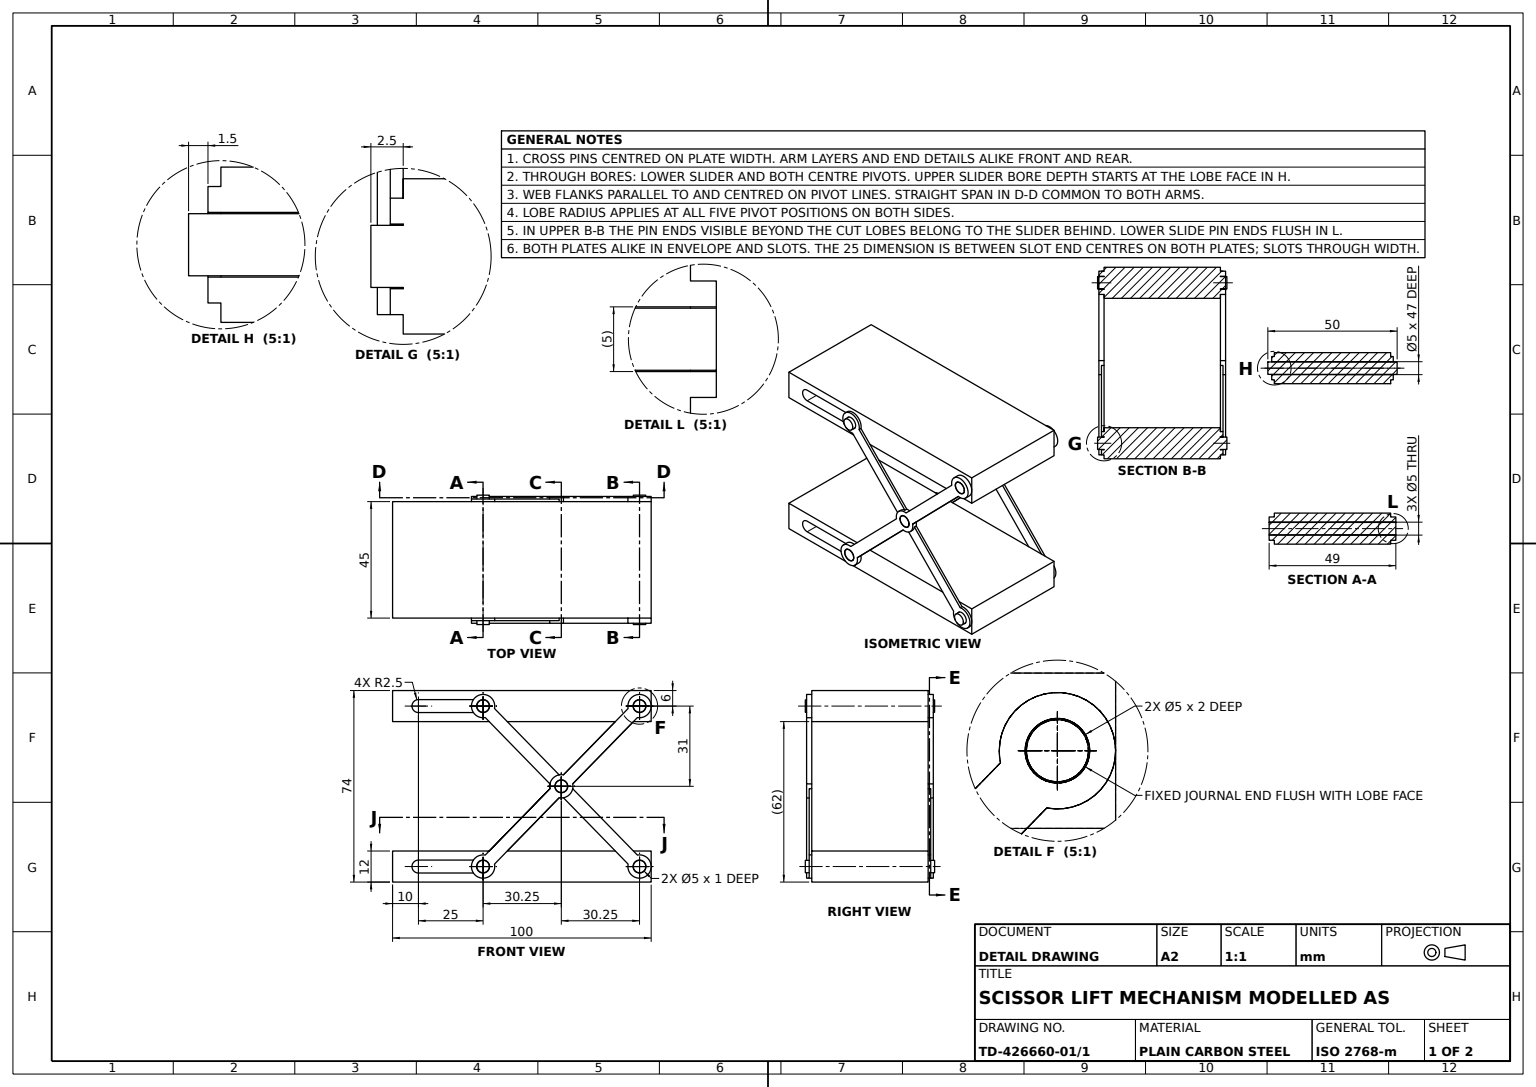
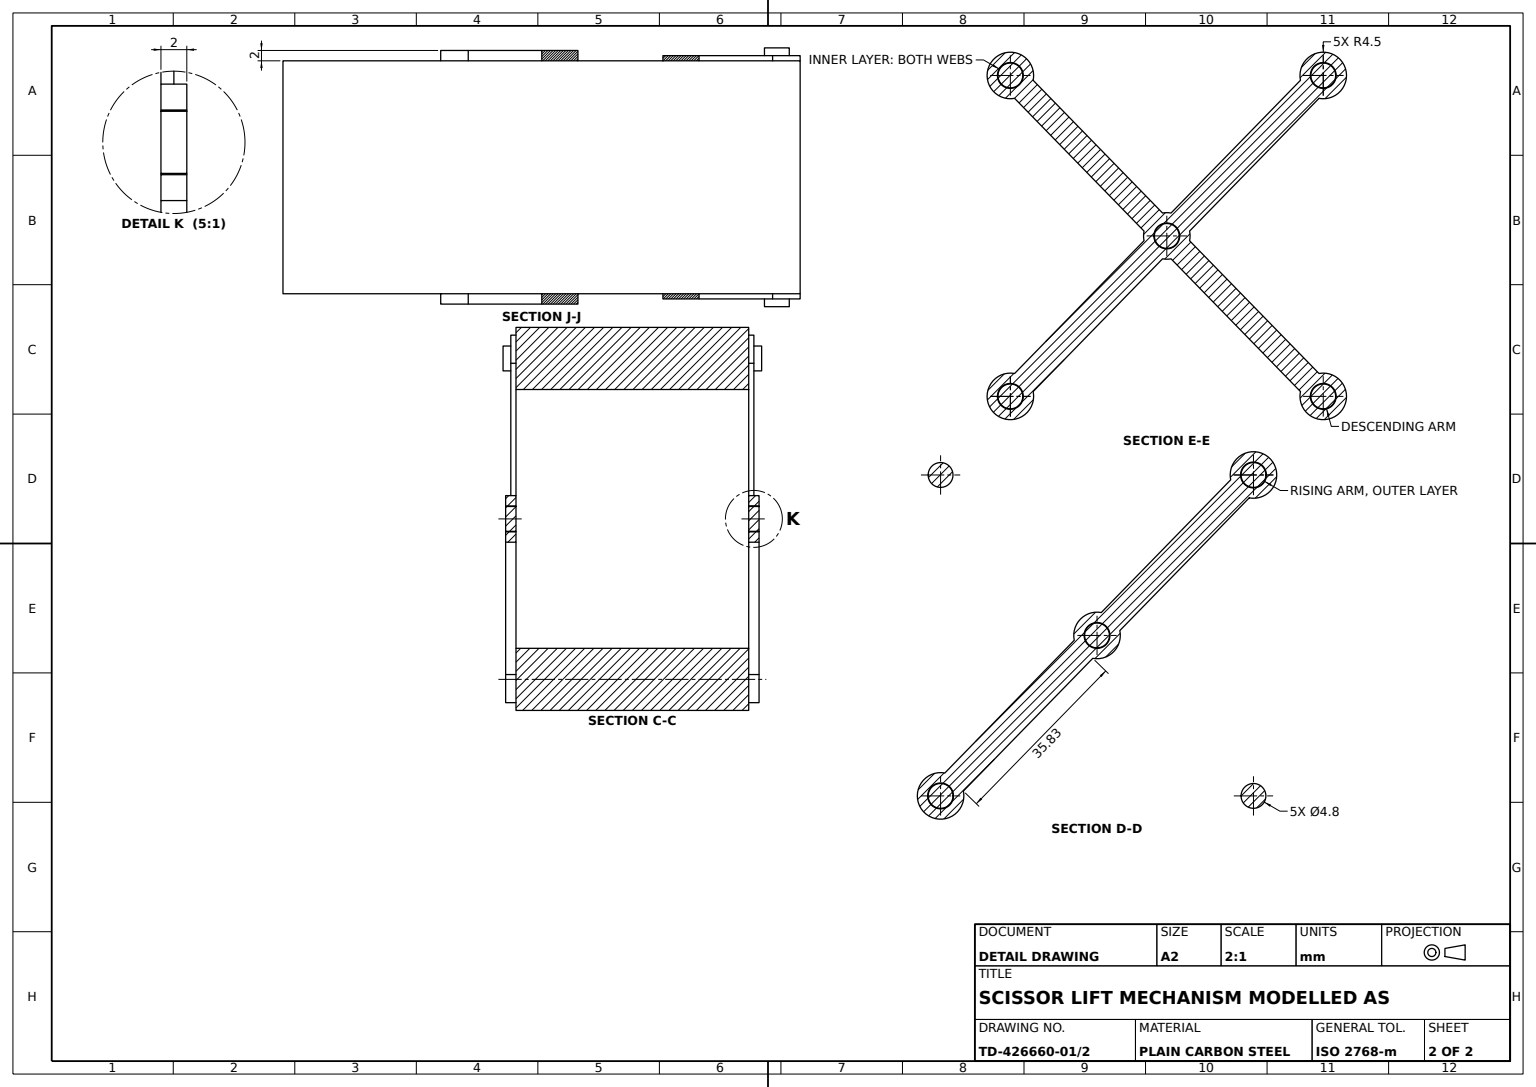
from build123d import *
from build123d.topology import SkipClean

# Parameters (mm, degrees)
BASE_PLATE_SKETCH_W              = 100
BASE_PLATE_SKETCH_H              = 45
BASE_PLATE_DEPTH                 = 12
BASE_PLATE_GUIDE_SLOT_DEPTH      = 200
TOP_PLATE_SKETCH_W               = 100
TOP_PLATE_SKETCH_H               = 45
TOP_PLATE_DEPTH                  = 12
TOP_PLATE_GUIDE_SLOT_DEPTH       = 50
FRONT_SCISSOR_ARM_A_SKETCH_R     = 2.5
FRONT_SCISSOR_ARM_A_DEPTH        = 1
FRONT_SCISSOR_ARM_B_SKETCH_R     = 2.5
FRONT_SCISSOR_ARM_B_DEPTH        = 2
FRONT_START                      = -2
FRONT_ARM_LINK_PIN_SKETCH_R      = 4.5
FRONT_ARM_LINK_PIN_SKETCH_R_2    = 2.5
FRONT_ARM_LINK_PIN_DEPTH         = 2
CENTER_PIVOT_PIN_FRONT_SKETCH_R  = 2.4
CENTER_PIVOT_PIN_FRONT_4_8_DEPTH = 2
LOWER_CROSS_PIN_SKETCH_R         = 2.4
LOWER_CROSS_PIN_4_8X49_DEPTH     = 49
UPPER_CROSS_PIN_HEAD_SKETCH_R    = 2.4
UPPER_CROSS_PIN_HEAD_DEPTH       = 1.5
UPPER_CROSS_PIN_SKETCH_R         = 2.4
UPPER_CROSS_PIN_4_8X47_5_DEPTH   = 47.5
FRONT_ARM_PIN_SKETCH_R           = 2.4
FRONT_ARM_PIN_4_8_DEPTH          = 2
LOWER_ROLLER_PIN_SKETCH_R        = 2.4
LOWER_ROLLER_PIN_4_8_DEPTH       = 2.5
REAR_START                       = 1
REAR_SCISSOR_ARM_A_SKETCH_R      = 2.5
REAR_SCISSOR_ARM_A_DEPTH         = 1
UPPER_START                      = 2.5
UPPER_CROSS_PIN_END_SKETCH_R     = 2.4
UPPER_CROSS_PIN_END_4_8_DEPTH    = 2.5
REAR_START_2                     = 2
REAR_SCISSOR_ARM_B_SKETCH_R      = 2.5
REAR_SCISSOR_ARM_B_DEPTH         = 2
CENTER_PIVOT_PIN_REAR_SKETCH_R   = 2.4
CENTER_PIVOT_PIN_REAR_4_8_DEPTH  = 2
REAR_ARM_PIN_SKETCH_R            = 2.4
REAR_ARM_PIN_4_8_DEPTH           = 2


with BuildPart() as part:
    # Base Plate Sketch → Base Plate (new body)
    with BuildSketch(Plane(origin=(0, 0, 0), x_dir=(1, 0, 0), z_dir=(0, 1, 0))):
        Rectangle(BASE_PLATE_SKETCH_W, BASE_PLATE_SKETCH_H)
    extrude(amount=BASE_PLATE_DEPTH)

    # Base Plate Guide Slot Sketch → Base Plate Guide Slot (cut)
    with BuildSketch(Plane.XY.offset(22.5)):
        with BuildLine():
            Line((-15, 3.5), (-40, 3.5))
            ThreePointArc((-40, 3.5), (-42.5, 6), (-40, 8.5))
            Line((-40, 8.5), (-15, 8.5))
            ThreePointArc((-15, 8.5), (-12.5, 6), (-15, 3.5))
        make_face()
    extrude(amount=-BASE_PLATE_GUIDE_SLOT_DEPTH, mode=Mode.SUBTRACT)



with BuildPart() as body_2:
    # Top Plate Sketch → Top Plate (new body)
    with BuildSketch(Plane(origin=(0, 62, 0), x_dir=(1, 0, 0), z_dir=(0, 1, 0))):
        Rectangle(TOP_PLATE_SKETCH_W, TOP_PLATE_SKETCH_H)
    extrude(amount=TOP_PLATE_DEPTH)

    # Top Plate Guide Slot Sketch → Top Plate Guide Slot (cut)
    with BuildSketch(Plane.XY.offset(22.5)):
        with BuildLine():
            Line((-15, 65.5), (-40, 65.5))
            ThreePointArc((-40, 65.5), (-42.5, 68), (-40, 70.5))
            Line((-40, 70.5), (-15, 70.5))
            ThreePointArc((-15, 70.5), (-12.5, 68), (-15, 65.5))
        make_face()
    extrude(amount=-TOP_PLATE_GUIDE_SLOT_DEPTH, mode=Mode.SUBTRACT)


with BuildPart() as part_1:
    with SkipClean():  # the faces are left unmerged after this step: merging them gives an invalid solid
        add(part.part)

        add(body_2.part)  # Front Scissor Arm A merges body 2
        # Front Scissor Arm A Sketch → Front Scissor Arm A (add)
        with BuildSketch(Plane.XY.offset(22.5)):
            with BuildLine():
                Line((-14.176120486, 63.576062552), (10.847562598, 37.931957574))
                ThreePointArc((10.847562598, 37.931957574), (12.029297901, 33.857218113), (16.073879514, 32.576062552))
                Line((16.073879514, 32.576062552), (41.097562598, 6.931957574))
                ThreePointArc((41.097562598, 6.931957574), (48.642781887, 2.779297901), (44.676120486, 10.423937448))
                Line((44.676120486, 10.423937448), (19.652437402, 36.068042426))
                ThreePointArc((19.652437402, 36.068042426), (18.470702099, 40.142781887), (14.426120486, 41.423937448))
                Line((14.426120486, 41.423937448), (-10.597562598, 67.068042426))
                ThreePointArc((-10.597562598, 67.068042426), (-18.142781887, 71.220702099), (-14.176120486, 63.576062552))
            make_face()
            with Locations(Location((-15, 68, 0), (0, 0, 270))):
                Circle(FRONT_SCISSOR_ARM_A_SKETCH_R, mode=Mode.SUBTRACT)
            with Locations((45.5, 6)):
                Circle(FRONT_SCISSOR_ARM_A_SKETCH_R, mode=Mode.SUBTRACT)
            with Locations((15.25, 37)):
                Circle(FRONT_SCISSOR_ARM_A_SKETCH_R, mode=Mode.SUBTRACT)
        extrude(amount=FRONT_SCISSOR_ARM_A_DEPTH)

    # Front Scissor Arm B Sketch → Front Scissor Arm B (add)
    with SkipClean():  # the faces are left unmerged after this step: merging them gives an invalid solid
        with BuildSketch(Plane.XY.offset(22.5)):
            with BuildLine():
                Line((16.073879514, 41.423937448), (41.097562598, 67.068042426))
                ThreePointArc((41.097562598, 67.068042426), (48.642781887, 71.220702099), (44.676120486, 63.576062552))
                Line((44.676120486, 63.576062552), (19.652437402, 37.931957574))
                ThreePointArc((19.652437402, 37.931957574), (18.470702099, 33.857218113), (14.426120486, 32.576062552))
                Line((14.426120486, 32.576062552), (-10.597562598, 6.931957574))
                ThreePointArc((-10.597562598, 6.931957574), (-18.142781887, 2.779297901), (-14.176120486, 10.423937448))
                Line((-14.176120486, 10.423937448), (10.847562598, 36.068042426))
                ThreePointArc((10.847562598, 36.068042426), (12.029297901, 40.142781887), (16.073879514, 41.423937448))
            make_face()
            with Locations((-15, 6)):
                Circle(FRONT_SCISSOR_ARM_B_SKETCH_R, mode=Mode.SUBTRACT)
            with Locations((45.5, 68)):
                Circle(FRONT_SCISSOR_ARM_B_SKETCH_R, mode=Mode.SUBTRACT)
            with Locations((15.25, 37)):
                Circle(FRONT_SCISSOR_ARM_B_SKETCH_R, mode=Mode.SUBTRACT)
        extrude(amount=FRONT_SCISSOR_ARM_B_DEPTH)

    # Front Arm Link Pin Sketch → Front Arm Link Pin (add)
    with SkipClean():  # the faces are left unmerged after this step: merging them gives an invalid solid
        with BuildSketch(Plane.XY.offset(24.5).offset(FRONT_START)):
            with Locations((15.25, 37)):
                Circle(FRONT_ARM_LINK_PIN_SKETCH_R)
            with Locations((15.25, 37)):
                Circle(FRONT_ARM_LINK_PIN_SKETCH_R_2, mode=Mode.SUBTRACT)
        extrude(amount=FRONT_ARM_LINK_PIN_DEPTH)

    # Front Arm Pin Sketch → Front Arm Pin Ø4.8 (add)
    with SkipClean():  # the faces are left unmerged after this step: merging them gives an invalid solid
        with BuildSketch(Plane.XY.offset(22.5)):
            with Locations(Location((45.5, 68, 0), (0, 0, 180))):
                Circle(FRONT_ARM_PIN_SKETCH_R)
        extrude(amount=FRONT_ARM_PIN_4_8_DEPTH)

    # Lower Roller Pin Sketch → Lower Roller Pin Ø4.8 (add)
    with SkipClean():  # the faces are left unmerged after this step: merging them gives an invalid solid
        with BuildSketch(Plane.XY.offset(22.5)):
            with Locations(Location((45.5, 6, 0), (0, 0, 180))):
                Circle(LOWER_ROLLER_PIN_SKETCH_R)
        extrude(amount=LOWER_ROLLER_PIN_4_8_DEPTH)

    # Rear Scissor Arm A Sketch → Rear Scissor Arm A (add)
    with BuildSketch(Plane(origin=(0, 0, -22.5), x_dir=(-1, 0, 0), z_dir=(0, 0, -1)).offset(REAR_START)):
        with BuildLine():
            Line((-14.426120486, 41.423937448), (10.597562598, 67.068042426))
            ThreePointArc((10.597562598, 67.068042426), (18.142781887, 71.220702099), (14.176120486, 63.576062552))
            Line((14.176120486, 63.576062552), (-10.847562598, 37.931957574))
            ThreePointArc((-10.847562598, 37.931957574), (-12.029297901, 33.857218113), (-16.073879514, 32.576062552))
            Line((-16.073879514, 32.576062552), (-41.097562598, 6.931957574))
            ThreePointArc((-41.097562598, 6.931957574), (-48.642781887, 2.779297901), (-44.676120486, 10.423937448))
            Line((-44.676120486, 10.423937448), (-19.652437402, 36.068042426))
            ThreePointArc((-19.652437402, 36.068042426), (-18.470702099, 40.142781887), (-14.426120486, 41.423937448))
        make_face()
        with Locations((15, 68)):
            Circle(REAR_SCISSOR_ARM_A_SKETCH_R, mode=Mode.SUBTRACT)
        with Locations(Location((-45.5, 6, 0), (0, 0, 180))):
            Circle(REAR_SCISSOR_ARM_A_SKETCH_R, mode=Mode.SUBTRACT)
        with Locations(Location((-15.25, 37, 0), (0, 0, 180))):
            Circle(REAR_SCISSOR_ARM_A_SKETCH_R, mode=Mode.SUBTRACT)
    extrude(amount=-REAR_SCISSOR_ARM_A_DEPTH)



with BuildPart() as body_2_2:
    # Center Pivot Pin Front Sketch → Center Pivot Pin Front Ø4.8 (new body)
    with BuildSketch(Plane.XY.offset(24.5)):
        with Locations((15.25, 37)):
            Circle(CENTER_PIVOT_PIN_FRONT_SKETCH_R)
    extrude(amount=-CENTER_PIVOT_PIN_FRONT_4_8_DEPTH)


with BuildPart() as body_3:
    # Lower Cross Pin Sketch → Lower Cross Pin Ø4.8x49 (new body)
    with BuildSketch(Plane.XY.offset(24.5)):
        with Locations((-15, 6)):
            Circle(LOWER_CROSS_PIN_SKETCH_R)
    extrude(amount=-LOWER_CROSS_PIN_4_8X49_DEPTH)


with BuildPart() as body_4:
    # Upper Cross Pin Head Sketch → Upper Cross Pin Head (new body)
    with BuildSketch(Plane.XY.offset(23.5)):
        with Locations((-15, 68)):
            Circle(UPPER_CROSS_PIN_HEAD_SKETCH_R)
    extrude(amount=UPPER_CROSS_PIN_HEAD_DEPTH)

    # Upper Cross Pin Sketch → Upper Cross Pin Ø4.8x47.5 (add)
    with BuildSketch(Plane.XY.offset(25)):
        with Locations((-15, 68)):
            Circle(UPPER_CROSS_PIN_SKETCH_R)
    extrude(amount=-UPPER_CROSS_PIN_4_8X47_5_DEPTH)


with BuildPart() as part_2:
    add(part_1.part)

    add(body_4.part)  # Upper Cross Pin End Ø4.8 merges body 4
    # Upper Cross Pin End Sketch → Upper Cross Pin End Ø4.8 (add)
    with BuildSketch(Plane(origin=(0, 0, -22.5), x_dir=(-1, 0, 0), z_dir=(0, 0, -1)).offset(UPPER_START)):
        with Locations((15, 68)):
            Circle(UPPER_CROSS_PIN_END_SKETCH_R)
        with Locations((-45.5, 6)):
            Circle(UPPER_CROSS_PIN_END_SKETCH_R)
    extrude(amount=-UPPER_CROSS_PIN_END_4_8_DEPTH)

    # Rear Scissor Arm B Sketch → Rear Scissor Arm B (add)
    with SkipClean():  # the faces are left unmerged after this step: merging them gives an invalid solid
        with BuildSketch(Plane(origin=(0, 0, -22.5), x_dir=(-1, 0, 0), z_dir=(0, 0, -1)).offset(REAR_START_2)):
            with BuildLine():
                Line((-10.847562598, 36.068042426), (14.176120486, 10.423937448))
                ThreePointArc((14.176120486, 10.423937448), (18.142781887, 2.779297901), (10.597562598, 6.931957574))
                Line((10.597562598, 6.931957574), (-14.426120486, 32.576062552))
                ThreePointArc((-14.426120486, 32.576062552), (-18.470702099, 33.857218113), (-19.652437402, 37.931957574))
                Line((-19.652437402, 37.931957574), (-44.676120486, 63.576062552))
                ThreePointArc((-44.676120486, 63.576062552), (-48.642781887, 71.220702099), (-41.097562598, 67.068042426))
                Line((-41.097562598, 67.068042426), (-16.073879514, 41.423937448))
                ThreePointArc((-16.073879514, 41.423937448), (-12.029297901, 40.142781887), (-10.847562598, 36.068042426))
            make_face()
            with Locations(Location((-45.5, 68, 0), (0, 0, 180))):
                Circle(REAR_SCISSOR_ARM_B_SKETCH_R, mode=Mode.SUBTRACT)
            with Locations(Location((15, 6, 0), (0, 0, 180))):
                Circle(REAR_SCISSOR_ARM_B_SKETCH_R, mode=Mode.SUBTRACT)
            with Locations(Location((-15.25, 37, 0), (0, 0, 180))):
                Circle(REAR_SCISSOR_ARM_B_SKETCH_R, mode=Mode.SUBTRACT)
        extrude(amount=-REAR_SCISSOR_ARM_B_DEPTH)

    # Rear Arm Pin Sketch → Rear Arm Pin Ø4.8 (add)
    with SkipClean():  # the faces are left unmerged after this step: merging them gives an invalid solid
        with BuildSketch(Plane(origin=(0, 0, -22.5), x_dir=(-1, 0, 0), z_dir=(0, 0, -1)).offset(REAR_START_2)):
            with Locations((-45.5, 68)):
                Circle(REAR_ARM_PIN_SKETCH_R)
        extrude(amount=-REAR_ARM_PIN_4_8_DEPTH)


with BuildPart() as body_4_2:
    # Center Pivot Pin Rear Sketch → Center Pivot Pin Rear Ø4.8 (new body)
    with BuildSketch(Plane(origin=(0, 0, -24.5), x_dir=(-1, 0, 0), z_dir=(0, 0, -1))):
        with Locations((-15.25, 37)):
            Circle(CENTER_PIVOT_PIN_REAR_SKETCH_R)
    extrude(amount=-CENTER_PIVOT_PIN_REAR_4_8_DEPTH)


solid = Compound([body_2_2.part, body_3.part, part_2.part, body_4_2.part])
